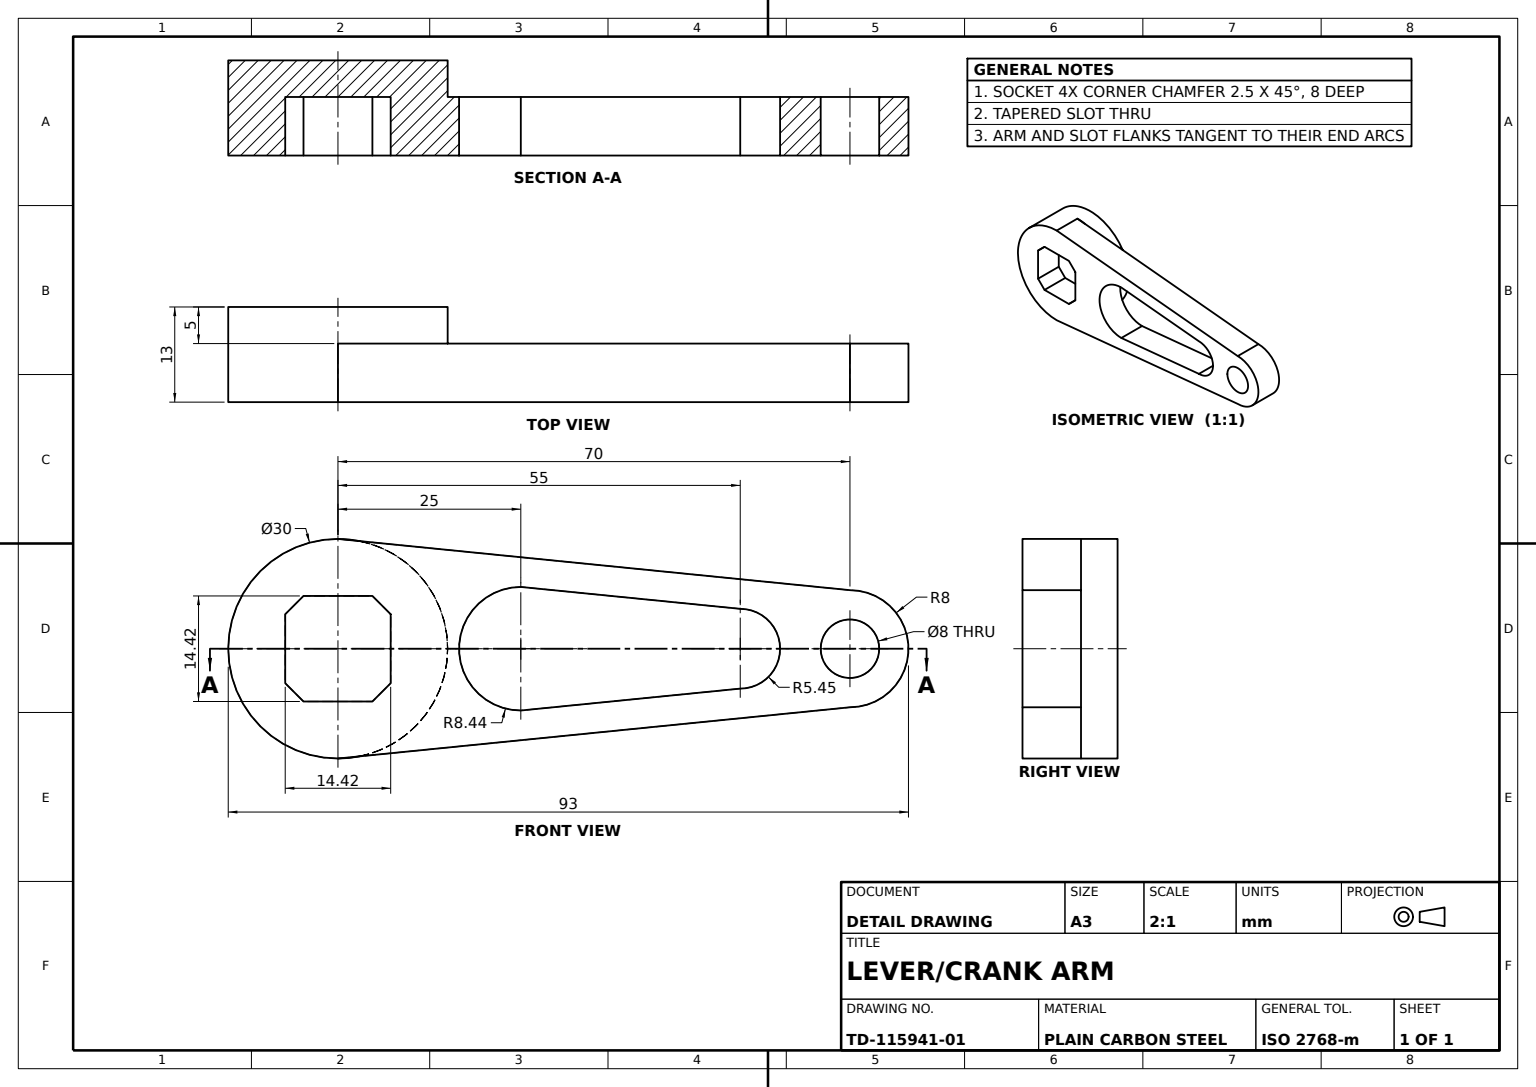
from build123d import *

# Parameters (mm, degrees)
LEVER_ARM_PLATE_DEPTH  = 8
TAPERED_SLOT_CUT_DEPTH = 8
HUB_START              = 5
HUB_BOSS_SKETCH_R      = 15
HUB_BOSS_DEPTH         = 5
PIN_HOLE_SKETCH_R      = 4
PIN_HOLE_DEPTH         = 8
HEX_SOCKET_CUT_DEPTH   = 8


with BuildPart() as part:
    # Lever Profile Sketch → Lever Arm Plate (new body)
    with BuildSketch(Plane.XY):
        with BuildLine():
            Line((0, 15), (70, 8))
            ThreePointArc((70, 8), (78, 0), (70, -8))
            Line((70, -8), (0, -15))
            ThreePointArc((0, -15), (-15, 0), (0, 15))
        make_face()
    extrude(amount=LEVER_ARM_PLATE_DEPTH)

    # Tapered Slot Sketch → Tapered Slot Cut (cut)
    with BuildSketch(Plane.XY.offset(8)):
        with BuildLine():
            Line((25, 8.44), (55, 5.45))
            ThreePointArc((55, 5.45), (60.45, 0), (55, -5.45))
            Line((55, -5.45), (25, -8.44))
            ThreePointArc((25, -8.44), (16.56, 0), (25, 8.44))
        make_face()
    extrude(amount=-TAPERED_SLOT_CUT_DEPTH, mode=Mode.SUBTRACT)

    # Hub Boss Sketch → Hub Boss (add)
    with BuildSketch(Plane(origin=(0, 0, 0), x_dir=(-1, 0, 0), z_dir=(0, 0, -1)).offset(HUB_START)):
        Circle(HUB_BOSS_SKETCH_R)
    extrude(amount=-HUB_BOSS_DEPTH)

    # Pin Hole Sketch → Pin Hole (cut)
    with BuildSketch(Plane.XY.offset(8)):
        with Locations((70, 0)):
            Circle(PIN_HOLE_SKETCH_R)
    extrude(amount=-PIN_HOLE_DEPTH, mode=Mode.SUBTRACT)

    # Hex Socket Sketch → Hex Socket Cut (cut)
    with BuildSketch(Plane.XY.offset(8)):
        Polygon((0, 7.21), (-4.71, 7.21), (-7.21, 4.71), (-7.21, -4.71), (-4.71, -7.21), (4.71, -7.21), (7.21, -4.71), (7.21, 4.71), (4.71, 7.21), align=None)
    extrude(amount=-HEX_SOCKET_CUT_DEPTH, mode=Mode.SUBTRACT)


solid = part.part
